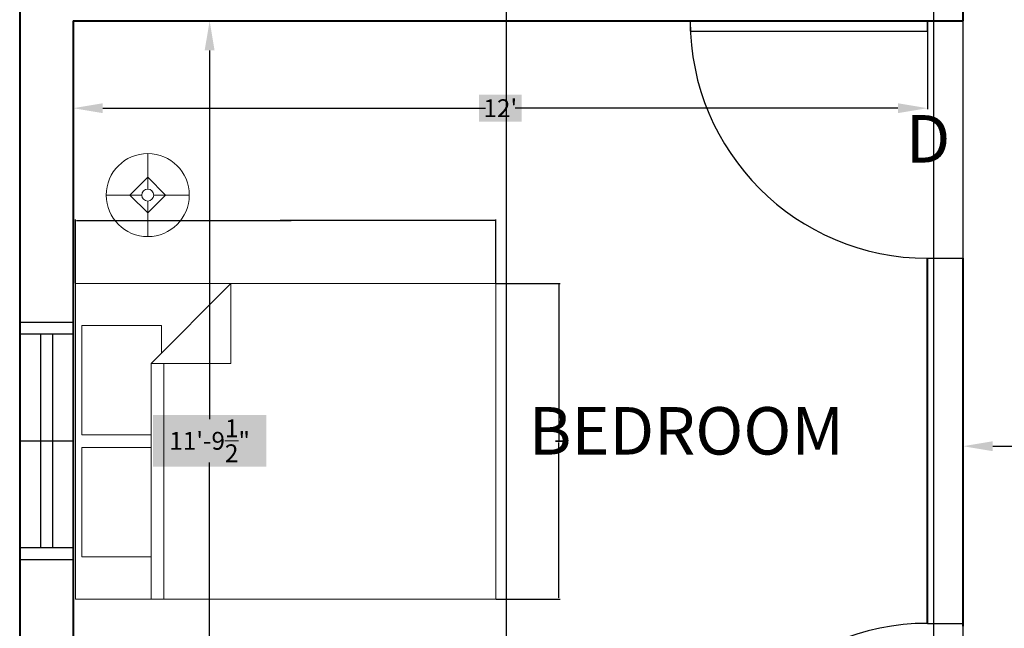
# Model space of a CAD drawing. Units: inches. Extents: x -301 to 715, y -607 to 364.
# Tile 66 of 141: x -205 to -39, y -176 to -73. Entities that reach past the tile are written whole.
import ezdxf

# ---------------------------------------------------------------- set-up
doc = ezdxf.new("R2010")
doc.units = ezdxf.units.IN
doc.header["$MEASUREMENT"] = 0
for name, color, linetype, lineweight in [('A-ANNO-DIMS', 2, 'Continuous', 18), ('A-ANNO-TEXT', 4, 'Continuous', 18), ('A-AREA-IDEN', 220, 'Continuous', 25), ('A-DOOR', 4, 'Continuous', 25), ('A-FURN', 8, 'Continuous', 18), ('A-GLAZ', 2, 'Continuous', 25), ('A-WALL', 3, 'Continuous', 40)]:
    doc.layers.add(name, color=color, linetype=linetype, lineweight=lineweight)
doc.styles.get("Standard").update_dxf_attribs({"font": 'arial.ttf'})
doc.dimstyles.get("Standard").update_dxf_attribs({"dimtxt": 0.18, "dimasz": 0.18, "dimexe": 0.18, "dimexo": 0.0625, "dimgap": 0.09, "dimtad": 0, "dimtih": 1, "dimtoh": 1, "dimdec": 1, "dimzin": 0, "dimdsep": 46, "dimlunit": 4, "dimtxsty": 'Standard', "dimcen": 0.09, "dimclrd": 3, "dimclre": 4, "dimclrt": 6, "dimadec": 0, "dimazin": 0, "dimtfac": 1, "dimtdec": 1, "dimtofl": 0, "dimtmove": 0, "dimatfit": 3, "dimfxl": 1, "dimtfill": 2, "dimtfillclr": 51, "dimtolj": 1, "dimtzin": 0, "dimarcsym": 0})

# ---------------------------------------------------------------- blocks, each defined once
blk = doc.blocks.new('*U4')
for p, q in [((0, 0), (0, -6)), ((40, 0), (40, -6))]:
    blk.add_line(p, q)
blk.add_lwpolyline([(0, 0), (0, 40), (1.75, 40), (1.75, 0)], close=True)
blk.add_arc((0, 0), 40, 0, 90)
blk = doc.blocks.new('*U5')
for p, q in [((0, 0), (0, -6)), ((-40, 0), (-40, -6))]:
    blk.add_line(p, q)
blk.add_lwpolyline([(0, 0), (0, 40), (-1.75, 40), (-1.75, 0)], close=True)
blk.add_arc((0, 0), 40, 90, 180)
blk = doc.blocks.new('Bed - Queen')
for p, q in [((0, -80.00003), (0, 0)), ((0, 0), (59.99999, 0)), ((59.99999, 0), (59.99999, -80.00003)), ((7.99999, -1.2), (28.79998, -1.2)), ((7.99999, -14.4), (7.99999, -1.2)), ((28.79998, -1.2), (28.79998, -14.4)), ((31.19999, -1.2), (51.99999, -1.2)), ((31.19999, -14.4), (31.19999, -1.2)), ((51.99999, -1.2), (51.99999, -16.4)), ((0, -14.4), (44.8, -14.4)), ((59.99999, -29.6), (44.8, -14.4)), ((44.8, -14.4), (44.8, -29.6)), ((44.8, -16.8), (0, -16.8)), ((51.99999, -16.4), (46.79936, -16.4)), ((44.8, -29.6), (59.99999, -29.6)), ((59.99999, -80.00003), (0, -80.00003))]:
    blk.add_line(p, q)
blk = doc.blocks.new('Lamp - Table')
for p, q in [((0, 7), (0, 1)), ((0, 3), (-3, 0)), ((3, 0), (0, 3)), ((-1, 0), (-7, 0)), ((-3, 0), (0, -3)), ((0, -3), (3, 0)), ((1, 0), (7, 0)), ((0, -1), (0, -7))]:
    blk.add_line(p, q)
for radius in [7, 1]:
    blk.add_circle((0, 0), radius)
blk = doc.blocks.new('*D40')
at = {"layer": 'A-ANNO-DIMS', "color": 0, "lineweight": -2, "transparency": 16777216}
for p, q in [((-195.6, -73.38), (-195.6, -88.22)), ((-51.6, -73.38), (-51.6, -88.22)), ((-190.6, -88.04), (-126.1, -88.04)), ((-56.6, -88.04), (-121.11, -88.04))]:
    blk.add_line(p, q, dxfattribs=at)
at = {"layer": 'A-ANNO-DIMS', "color": 0, "transparency": 16777216}
for points in [[(-190.6, -87.21), (-190.6, -88.87), (-195.6, -88.04)], [(-56.6, -87.21), (-56.6, -88.87), (-51.6, -88.04)]]:
    blk.add_solid(points, dxfattribs=at)
at = {"layer": 'Defpoints', "color": 0, "transparency": 16777216}
for p in [(-195.6, -73.32), (-51.6, -73.32), (-51.6, -88.04)]:
    blk.add_point(p, dxfattribs=at)
at = {"layer": 'A-ANNO-DIMS', "color": 0, "transparency": 16777216, "insert": (-123.6, -88.04), "char_height": 3, "attachment_point": 5, "bg_fill": 1, "box_fill_scale": 1.25, "bg_fill_color": 51, "bg_fill_transparency": 0}
blk.add_mtext("\\A1;12'", dxfattribs=at)
blk = doc.blocks.new('*D41')
at = {"layer": 'A-ANNO-DIMS', "color": 0, "lineweight": -2, "transparency": 16777216}
for p, q in [((-195.54, -73.32), (-172.41, -73.32)), ((-172.59, -78.32), (-172.59, -140.44)), ((-172.59, -209.82), (-172.59, -147.7)), ((-195.54, -214.82), (-172.41, -214.82))]:
    blk.add_line(p, q, dxfattribs=at)
at = {"layer": 'A-ANNO-DIMS', "color": 0, "transparency": 16777216}
for points in [[(-173.43, -78.32), (-171.76, -78.32), (-172.59, -73.32)], [(-173.43, -209.82), (-171.76, -209.82), (-172.59, -214.82)]]:
    blk.add_solid(points, dxfattribs=at)
at = {"layer": 'Defpoints', "color": 0, "transparency": 16777216}
for p in [(-195.6, -73.32), (-195.6, -214.82), (-172.59, -214.82)]:
    blk.add_point(p, dxfattribs=at)
at = {"layer": 'A-ANNO-DIMS', "color": 0, "transparency": 16777216, "insert": (-172.59, -144.07), "char_height": 3, "attachment_point": 5, "bg_fill": 1, "box_fill_scale": 1.25, "bg_fill_color": 51, "bg_fill_transparency": 0}
blk.add_mtext('\\A1;11\'-9{\\H1x;\\S1/2;}"', dxfattribs=at)
blk = doc.blocks.new('*D42')
at = {"layer": 'A-ANNO-DIMS', "color": 0, "lineweight": -2, "transparency": 16777216}
for p, q in [((-45.6, -130.88), (-45.6, -145.16)), ((123.9, -130.88), (123.9, -145.16)), ((-40.6, -144.98), (32.95, -144.98)), ((118.9, -144.98), (45.34, -144.98))]:
    blk.add_line(p, q, dxfattribs=at)
at = {"layer": 'A-ANNO-DIMS', "color": 0, "transparency": 16777216}
for points in [[(-40.6, -144.15), (-40.6, -145.82), (-45.6, -144.98)], [(118.9, -144.15), (118.9, -145.82), (123.9, -144.98)]]:
    blk.add_solid(points, dxfattribs=at)
at = {"layer": 'Defpoints', "color": 0, "transparency": 16777216}
for p in [(-45.6, -130.82), (123.9, -130.82), (-45.6, -144.98)]:
    blk.add_point(p, dxfattribs=at)
at = {"layer": 'A-ANNO-DIMS', "color": 0, "transparency": 16777216, "insert": (39.15, -144.98), "char_height": 3, "attachment_point": 5, "bg_fill": 1, "box_fill_scale": 1.25, "bg_fill_color": 51, "bg_fill_transparency": 0}
blk.add_mtext('\\A1;14\'-1{\\H1x;\\S1/2;}"', dxfattribs=at)
blk = doc.blocks.new('WIN-36-PLAN')
for p, q in [((0, 0), (0, 9)), ((2, 0), (2, 9)), ((20, 0), (20, 9)), ((38, 0), (38, 9)), ((40, 0), (40, 9)), ((2, 5.5), (38, 5.5)), ((2, 3.5), (38, 3.5))]:
    blk.add_line(p, q)
blk = doc.blocks.new('*D108')
at = {"layer": 'A-ANNO-DIMS', "color": 4, "lineweight": -2, "transparency": 16777216}
for p, q in [((-195.21, -117.51), (-195.21, -106.77)), ((-124.35, -117.51), (-124.35, -106.77))]:
    blk.add_line(p, q, dxfattribs=at)
at = {"layer": 'A-ANNO-DIMS', "color": 3, "lineweight": -2, "transparency": 16777216}
for p, q in [((-195.03, -106.95), (-160.78, -106.95)), ((-124.53, -106.95), (-158.78, -106.95))]:
    blk.add_line(p, q, dxfattribs=at)
at = {"layer": 'A-ANNO-DIMS', "color": 3, "transparency": 16777216}
for points in [[(-195.03, -106.92), (-195.03, -106.98), (-195.21, -106.95)], [(-124.53, -106.92), (-124.53, -106.98), (-124.35, -106.95)]]:
    blk.add_solid(points, dxfattribs=at)
at = {"layer": 'Defpoints', "color": 0, "transparency": 16777216}
for p in [(-195.21, -106.95), (-195.21, -117.57), (-124.35, -117.57)]:
    blk.add_point(p, dxfattribs=at)
at = {"layer": 'A-ANNO-DIMS', "color": 6, "transparency": 16777216, "insert": (-159.78, -106.95), "char_height": 0.18, "attachment_point": 5, "bg_fill": 1, "box_fill_scale": 1.25, "bg_fill_color": 51, "bg_fill_transparency": 0}
blk.add_mtext('\\A1;BED 5\'-11" TYP.', dxfattribs=at)
blk = doc.blocks.new('*D109')
at = {"layer": 'A-ANNO-DIMS', "color": 4, "lineweight": -2, "transparency": 16777216}
for p, q in [((-124.29, -117.57), (-113.54, -117.57)), ((-124.29, -170.72), (-113.54, -170.72))]:
    blk.add_line(p, q, dxfattribs=at)
at = {"layer": 'A-ANNO-DIMS', "color": 3, "lineweight": -2, "transparency": 16777216}
for p, q in [((-113.72, -117.75), (-113.72, -143.96)), ((-113.72, -170.54), (-113.72, -144.33))]:
    blk.add_line(p, q, dxfattribs=at)
at = {"layer": 'A-ANNO-DIMS', "color": 3, "transparency": 16777216}
for points in [[(-113.75, -117.75), (-113.69, -117.75), (-113.72, -117.57)], [(-113.75, -170.54), (-113.69, -170.54), (-113.72, -170.72)]]:
    blk.add_solid(points, dxfattribs=at)
at = {"layer": 'Defpoints', "color": 0, "transparency": 16777216}
for p in [(-124.35, -117.57), (-113.72, -117.57), (-124.35, -170.72)]:
    blk.add_point(p, dxfattribs=at)
at = {"layer": 'A-ANNO-DIMS', "color": 6, "transparency": 16777216, "insert": (-113.72, -144.14), "char_height": 0.18, "attachment_point": 5, "bg_fill": 1, "box_fill_scale": 1.25, "bg_fill_color": 51, "bg_fill_transparency": 0}
blk.add_mtext('\\A1;4\'-5" TYP.', dxfattribs=at)
blk = doc.blocks.new('*D151')
at = {"layer": 'A-ANNO-DIMS', "color": 4, "lineweight": -2, "transparency": 16777216}
for p, q in [((-204.6, -223.76), (-204.6, 359.61)), ((-45.6, -214.76), (-45.6, 359.61))]:
    blk.add_line(p, q, dxfattribs=at)
at = {"layer": 'A-ANNO-DIMS', "color": 3, "lineweight": -2, "transparency": 16777216}
for p, q in [((-204.42, 359.43), (-125.49, 359.43)), ((-45.78, 359.43), (-124.71, 359.43))]:
    blk.add_line(p, q, dxfattribs=at)
at = {"layer": 'A-ANNO-DIMS', "color": 3, "transparency": 16777216}
for points in [[(-204.42, 359.46), (-204.42, 359.4), (-204.6, 359.43)], [(-45.78, 359.46), (-45.78, 359.4), (-45.6, 359.43)]]:
    blk.add_solid(points, dxfattribs=at)
at = {"layer": 'Defpoints', "color": 0, "transparency": 16777216}
for p in [(-45.6, 359.43), (-45.6, -214.82), (-204.6, -223.82)]:
    blk.add_point(p, dxfattribs=at)
at = {"layer": 'A-ANNO-DIMS', "color": 6, "transparency": 16777216, "insert": (-125.1, 359.43), "char_height": 0.18, "attachment_point": 5, "bg_fill": 1, "box_fill_scale": 1.25, "bg_fill_color": 51, "bg_fill_transparency": 0}
blk.add_mtext('\\A1;13\'-3"', dxfattribs=at)
blk = doc.blocks.new('*D158')
at = {"layer": 'A-ANNO-DIMS', "color": 4, "lineweight": -2, "transparency": 16777216}
for p, q in [((-122.6, 221.62), (-122.6, -296.87)), ((-50.6, 221.62), (-50.6, -296.87))]:
    blk.add_line(p, q, dxfattribs=at)
at = {"layer": 'A-ANNO-DIMS', "color": 3, "lineweight": -2, "transparency": 16777216}
for p, q in [((-122.42, -296.69), (-86.93, -296.69)), ((-50.78, -296.69), (-86.27, -296.69))]:
    blk.add_line(p, q, dxfattribs=at)
at = {"layer": 'A-ANNO-DIMS', "color": 3, "transparency": 16777216}
for points in [[(-122.42, -296.66), (-122.42, -296.72), (-122.6, -296.69)], [(-50.78, -296.66), (-50.78, -296.72), (-50.6, -296.69)]]:
    blk.add_solid(points, dxfattribs=at)
at = {"layer": 'Defpoints', "color": 0, "transparency": 16777216}
for p in [(-122.6, 221.68), (-50.6, 221.68), (-50.6, -296.69)]:
    blk.add_point(p, dxfattribs=at)
at = {"layer": 'A-ANNO-DIMS', "color": 6, "transparency": 16777216, "insert": (-86.6, -296.69), "char_height": 0.18, "attachment_point": 5, "bg_fill": 1, "box_fill_scale": 1.25, "bg_fill_color": 51, "bg_fill_transparency": 0}
blk.add_mtext('\\A1;6\'-0"', dxfattribs=at)

msp = doc.modelspace()

# ---------------------------------------------------------------- linework, layer by layer
at = {"layer": 'A-WALL'}
for p, q in [((-45.6, -73.32), (-45.6, 25.68)), ((-204.6, -67.32), (-204.6, -223.82)), ((-195.6, -73.32), (-45.6, -73.32)), ((-195.6, -73.32), (-195.6, -214.82)), ((-51.6, -174.82), (-51.6, -113.32)), ((-45.6, -175.27), (-45.6, -113.32))]:
    msp.add_line(p, q, dxfattribs=at)

# ---------------------------------------------------------------- block references
at = {"layer": 'A-DOOR', "rotation": 90}
for name, p in [('*U5', (-51.6, -73.32)), ('*U4', (-51.6, -214.82))]:
    msp.add_blockref(name, p, dxfattribs=at)
at = {"layer": 'A-FURN'}
msp.add_blockref('Lamp - Table', (-183.02, -102.68), dxfattribs=at)
at = {"layer": 'A-FURN', "xscale": 0.8856750462000775, "yscale": 0.8856750462000775, "zscale": 0.8856750462000775, "rotation": 90}
msp.add_blockref('Bed - Queen', (-195.21, -170.72), dxfattribs=at)
at = {"layer": 'A-GLAZ', "rotation": 270.0000000000002}
msp.add_blockref('WIN-36-PLAN', (-204.6, -124.07), dxfattribs=at)

# ---------------------------------------------------------------- texts
at = {"layer": 'A-ANNO-TEXT'}
msp.add_text('D', height=8, dxfattribs=at).set_placement((-55.26, -97.2))
at = {"layer": 'A-AREA-IDEN', "insert": (-118.78, -138.39), "char_height": 8, "attachment_point": 1}
msp.add_mtext_dynamic_manual_height_columns('BEDROOM', width=73.06, gutter_width=1, heights=[0], dxfattribs=at)

# ---------------------------------------------------------------- dimensions: what is measured, and where the dimension line sits
at = {"layer": 'A-ANNO-DIMS'}
for base, p1, p2, override, picture, middle in [((-45.6, 359.43), (-204.6, -223.82), (-45.6, -214.82), {"dimdec": 1, "dimlfac": 1, "dimrnd": 0, "dimzin": 1, "dimdsep": 46, "dimlunit": 4, "dimfrac": 2}, '*D151', (-125.1, 359.43)), ((-50.6, -296.69), (-122.6, 221.68), (-50.6, 221.68), {"dimdec": 1, "dimlfac": 1, "dimrnd": 0, "dimzin": 1, "dimdsep": 46, "dimlunit": 4, "dimfrac": 2}, '*D158', (-86.6, -296.69)), ((-51.6, -88.04), (-195.6, -73.32), (-51.6, -73.32), {"dimtxt": 3, "dimasz": 5, "dimclrd": 0, "dimclre": 0, "dimclrt": 0}, '*D40', (-123.6, -88.04)), ((-45.6, -144.98), (123.9, -130.82), (-45.6, -130.82), {"dimtxt": 3, "dimasz": 5, "dimclrd": 0, "dimclre": 0, "dimclrt": 0}, '*D42', (39.15, -144.98))]:
    dim = msp.add_linear_dim(base=base, p1=p1, p2=p2, dimstyle='Standard', override=override, dxfattribs=at)
    dim.commit()
    dim.dimension.update_dxf_attribs({"geometry": picture, "text_midpoint": middle})
dim = msp.add_linear_dim(base=(-172.59, -214.82), p1=(-195.6, -73.32), p2=(-195.6, -214.82), angle=90, dimstyle='Standard', override={"dimtxt": 3, "dimasz": 5, "dimclrd": 0, "dimclre": 0, "dimclrt": 0}, dxfattribs=at)
dim.commit()
dim.dimension.update_dxf_attribs({"geometry": '*D41', "text_midpoint": (-172.59, -144.07)})
for base, p1, p2, angle, text, picture, middle in [((-195.21, -106.95), (-124.35, -117.57), (-195.21, -117.57), 180, 'BED <> TYP.', '*D108', (-159.78, -106.95)), ((-113.7244, -117.5746), (-124.3525, -170.7151), (-124.3525, -117.5746), 90, '<> TYP.', '*D109', (-113.7244, -144.1448))]:
    dim = msp.add_linear_dim(base=base, p1=p1, p2=p2, angle=angle, text=text, dimstyle='Standard', override={"dimdec": 1, "dimlfac": 1, "dimrnd": 0, "dimzin": 1, "dimdsep": 46, "dimlunit": 4, "dimfrac": 2}, dxfattribs=at)
    dim.commit()
    dim.dimension.update_dxf_attribs({"geometry": picture, "text_midpoint": middle})

doc.saveas('drawing.dxf')
